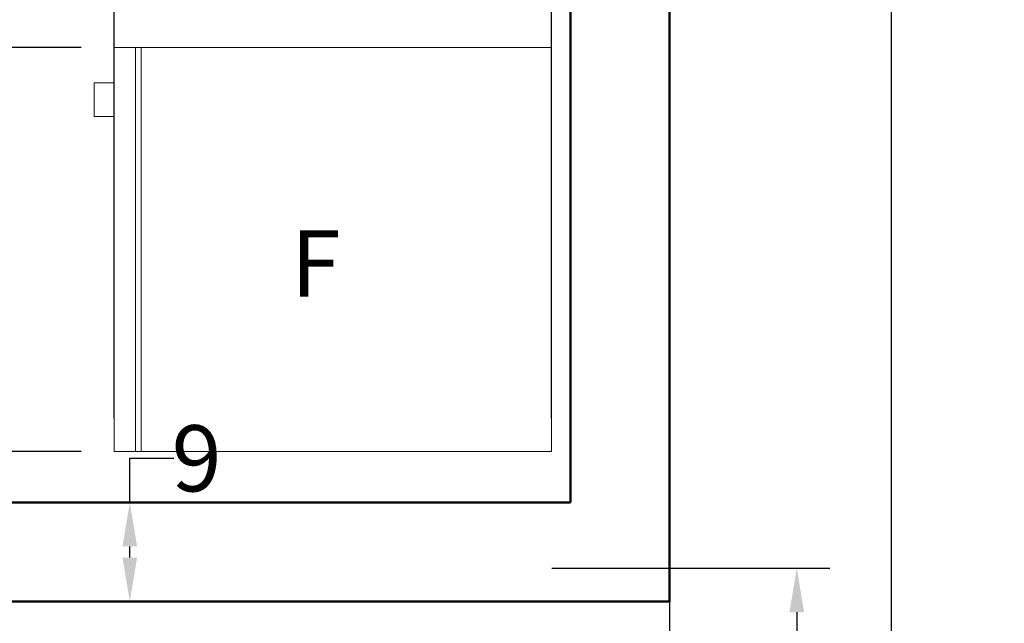
# Model space of a CAD drawing. Units: inches. Extents: x 89 to 490, y -59 to 378.
# Tile 17 of 20: x 400 to 490, y 3 to 58. Entities that reach past the tile are written whole.
import ezdxf

# ---------------------------------------------------------------- set-up
doc = ezdxf.new("R2010")
doc.units = ezdxf.units.IN
doc.header["$MEASUREMENT"] = 0
for name, color, linetype, lineweight in [('A-ANNO-DIMS', 2, 'Continuous', 18), ('A-ANNO-TEXT', 7, 'Continuous', 18), ('L-PLNT-EDGE', 31, 'Continuous', 25), ('Outer Walls', 12, 'Continuous', 50), ('Refrigerator', 40, 'Continuous', 18)]:
    doc.layers.add(name, color=color, linetype=linetype, lineweight=lineweight)
doc.styles.get("Standard").update_dxf_attribs({"font": 'arial.ttf'})
doc.dimstyles.get("Standard").update_dxf_attribs({"dimtxt": 6, "dimasz": 4, "dimexe": 3, "dimexo": 3, "dimgap": 0.09, "dimtad": 0, "dimtih": 1, "dimtoh": 1, "dimdec": 1, "dimzin": 0, "dimdsep": 46, "dimlunit": 3, "dimtxsty": 'Standard', "dimcen": 0.09, "dimadec": 0, "dimazin": 0, "dimtfac": 1, "dimtdec": 1, "dimtofl": 0, "dimtmove": 0, "dimatfit": 3, "dimfxl": 1, "dimtolj": 1, "dimtzin": 0, "dimarcsym": 0})

# ---------------------------------------------------------------- blocks, each defined once
blk = doc.blocks.new('*D37')
at = {"layer": 'A-ANNO-DIMS', "color": 0, "lineweight": -2, "transparency": 16777216}
for p, q in [((410.454, 13.741), (410.454, 17.741)), ((410.454, 17.741), (414.454, 17.741)), ((402.654, 13.741), (413.454, 13.741)), ((410.454, 8.741), (410.454, 9.741)), ((402.654, 4.741), (413.454, 4.741))]:
    blk.add_line(p, q, dxfattribs=at)
at = {"layer": 'A-ANNO-DIMS', "color": 0, "transparency": 16777216}
for points in [[(409.787, 9.741), (411.121, 9.741), (410.454, 13.741)], [(409.787, 8.741), (411.121, 8.741), (410.454, 4.741)]]:
    blk.add_solid(points, dxfattribs=at)
at = {"layer": 'Defpoints', "color": 0, "transparency": 16777216}
for p in [(399.654, 13.741), (410.454, 13.741), (399.654, 4.741)]:
    blk.add_point(p, dxfattribs=at)
at = {"layer": 'A-ANNO-DIMS', "color": 0, "transparency": 16777216, "insert": (416.517, 17.741), "char_height": 6, "attachment_point": 5}
blk.add_mtext('\\A1;9', dxfattribs=at)
blk = doc.blocks.new('*D47')
at = {"layer": 'A-ANNO-DIMS', "color": 0, "lineweight": -2, "transparency": 16777216}
for p, q in [((448.739, 7.78), (473.983, 7.78)), ((470.983, 3.78), (470.983, -5.387)), ((470.983, -20.866), (470.983, -11.698)), ((448.739, -24.866), (473.983, -24.866))]:
    blk.add_line(p, q, dxfattribs=at)
at = {"layer": 'A-ANNO-DIMS', "color": 0, "transparency": 16777216}
for points in [[(470.316, 3.78), (471.65, 3.78), (470.983, 7.78)], [(470.316, -20.866), (471.65, -20.866), (470.983, -24.866)]]:
    blk.add_solid(points, dxfattribs=at)
at = {"layer": 'Defpoints', "color": 0, "transparency": 16777216}
for p in [(445.739, 7.78), (470.983, 7.78), (445.739, -24.866)]:
    blk.add_point(p, dxfattribs=at)
at = {"layer": 'A-ANNO-DIMS', "color": 0, "transparency": 16777216, "insert": (470.983, -8.543), "char_height": 6, "attachment_point": 5}
blk.add_mtext('\\A1;33', dxfattribs=at)
blk = doc.blocks.new('*D48')
at = {"layer": 'A-ANNO-DIMS', "color": 0, "lineweight": -2, "transparency": 16777216}
for p, q in [((127.441, 10.741), (127.441, -49.809)), ((459.441, -29.659), (459.441, -49.809)), ((131.441, -46.809), (286.756, -46.809)), ((455.441, -46.809), (300.127, -46.809))]:
    blk.add_line(p, q, dxfattribs=at)
at = {"layer": 'A-ANNO-DIMS', "color": 0, "transparency": 16777216}
for points in [[(131.441, -46.143), (131.441, -47.476), (127.441, -46.809)], [(455.441, -46.143), (455.441, -47.476), (459.441, -46.809)]]:
    blk.add_solid(points, dxfattribs=at)
at = {"layer": 'Defpoints', "color": 0, "transparency": 16777216}
for p in [(127.441, 13.741), (459.441, -26.659), (459.441, -46.809)]:
    blk.add_point(p, dxfattribs=at)
at = {"layer": 'A-ANNO-DIMS', "color": 0, "transparency": 16777216, "insert": (293.441, -46.809), "char_height": 6, "attachment_point": 5}
blk.add_mtext('\\A1;332', dxfattribs=at)
blk = doc.blocks.new('*D49')
at = {"layer": 'A-ANNO-DIMS', "color": 0, "lineweight": -2, "transparency": 16777216}
for p, q in [((462.441, 353.741), (482.591, 353.741)), ((479.591, 349.741), (479.591, 166.696)), ((479.591, -22.659), (479.591, 160.385)), ((462.441, -26.659), (482.591, -26.659))]:
    blk.add_line(p, q, dxfattribs=at)
at = {"layer": 'A-ANNO-DIMS', "color": 0, "transparency": 16777216}
for points in [[(478.925, 349.741), (480.258, 349.741), (479.591, 353.741)], [(478.925, -22.659), (480.258, -22.659), (479.591, -26.659)]]:
    blk.add_solid(points, dxfattribs=at)
at = {"layer": 'Defpoints', "color": 0, "transparency": 16777216}
for p in [(459.441, 353.741), (479.591, 353.741), (459.441, -26.659)]:
    blk.add_point(p, dxfattribs=at)
at = {"layer": 'A-ANNO-DIMS', "color": 0, "transparency": 16777216, "insert": (479.591, 163.541), "char_height": 6, "attachment_point": 5}
blk.add_mtext('\\A1;380.4', dxfattribs=at)
blk = doc.blocks.new('*D64')
at = {"layer": 'A-ANNO-DIMS', "color": 0, "lineweight": -2, "transparency": 16777216}
for p, q in [((399.654, 16.741), (399.654, 376.891)), ((450.441, 16.741), (450.441, 376.891)), ((403.654, 373.891), (414.828, 373.891)), ((446.441, 373.891), (435.267, 373.891))]:
    blk.add_line(p, q, dxfattribs=at)
at = {"layer": 'A-ANNO-DIMS', "color": 0, "transparency": 16777216}
for points in [[(403.654, 374.558), (403.654, 373.225), (399.654, 373.891)], [(446.441, 374.558), (446.441, 373.225), (450.441, 373.891)]]:
    blk.add_solid(points, dxfattribs=at)
at = {"layer": 'Defpoints', "color": 0, "transparency": 16777216}
for p in [(450.441, 373.891), (399.654, 13.741), (450.441, 13.741)]:
    blk.add_point(p, dxfattribs=at)
at = {"layer": 'A-ANNO-DIMS', "color": 0, "transparency": 16777216, "insert": (425.048, 373.891), "char_height": 6, "attachment_point": 5}
blk.add_mtext('\\A1;50.79', dxfattribs=at)
blk = doc.blocks.new('*D71')
at = {"layer": 'A-ANNO-DIMS', "color": 0, "lineweight": -2, "transparency": 16777216}
for p, q in [((409.039, 21.374), (409.039, 376.891)), ((448.723, 21.374), (448.723, 376.891)), ((413.039, 373.891), (416.351, 373.891)), ((444.723, 373.891), (441.411, 373.891))]:
    blk.add_line(p, q, dxfattribs=at)
at = {"layer": 'A-ANNO-DIMS', "color": 0, "transparency": 16777216}
for points in [[(413.039, 374.558), (413.039, 373.225), (409.039, 373.891)], [(444.723, 374.558), (444.723, 373.225), (448.723, 373.891)]]:
    blk.add_solid(points, dxfattribs=at)
at = {"layer": 'Defpoints', "color": 0, "transparency": 16777216}
for p in [(448.723, 373.891), (409.039, 18.374), (448.723, 18.374)]:
    blk.add_point(p, dxfattribs=at)
at = {"layer": 'A-ANNO-DIMS', "color": 0, "transparency": 16777216, "insert": (428.881, 373.891), "char_height": 6, "attachment_point": 5}
blk.add_mtext('\\A1;39.684', dxfattribs=at)
blk = doc.blocks.new('*D72')
at = {"layer": 'A-ANNO-DIMS', "color": 0, "lineweight": -2, "transparency": 16777216}
for p, q in [((406.039, 55.006), (385.889, 55.006)), ((388.889, 51.006), (388.889, 39.845)), ((388.889, 22.374), (388.889, 33.534)), ((406.039, 18.374), (385.889, 18.374))]:
    blk.add_line(p, q, dxfattribs=at)
at = {"layer": 'A-ANNO-DIMS', "color": 0, "transparency": 16777216}
for points in [[(388.222, 51.006), (389.555, 51.006), (388.889, 55.006)], [(388.222, 22.374), (389.555, 22.374), (388.889, 18.374)]]:
    blk.add_solid(points, dxfattribs=at)
at = {"layer": 'Defpoints', "color": 0, "transparency": 16777216}
for p in [(388.889, 55.006), (409.039, 55.006), (409.039, 18.374)]:
    blk.add_point(p, dxfattribs=at)
at = {"layer": 'A-ANNO-DIMS', "color": 0, "transparency": 16777216, "insert": (388.889, 36.69), "char_height": 6, "attachment_point": 5}
blk.add_mtext('\\A1;36.63', dxfattribs=at)

msp = doc.modelspace()

# ---------------------------------------------------------------- linework, layer by layer
at = {"layer": 'L-PLNT-EDGE'}
msp.add_line((459.4414, 12.3406), (459.4414, -26.6594), dxfattribs=at)
at = {"layer": 'Outer Walls'}
for p, q in [((450.4414, 13.7413), (450.4414, 195.7413)), ((270.4414, 13.7413), (450.4414, 13.7413))]:
    msp.add_line(p, q, dxfattribs=at)
msp.add_lwpolyline([(214.6478, 67.7413), (265.4414, 67.7413), (265.4414, 4.7413), (459.4414, 4.7413), (459.4414, 353.7413), (127.4414, 353.7413), (127.4414, 13.7413)], dxfattribs=at)
at = {"layer": 'Refrigerator'}
for p, q in [((410.973, 18.3742), (410.973, 55.0057)), ((411.4809, 18.3742), (411.4809, 55.0057))]:
    msp.add_line(p, q, dxfattribs=at)
msp.add_lwpolyline([(448.7229, 55.0057), (448.7229, 18.3742), (409.0388, 18.3742), (409.0388, 55.0057)], close=True, dxfattribs=at)
msp.add_lwpolyline([(409.0388, 48.7515), (407.2072, 48.7515), (407.2072, 51.8041), (409.0388, 51.8041)], dxfattribs=at)

# ---------------------------------------------------------------- texts
at = {"layer": 'A-ANNO-TEXT', "insert": (425.065, 38.4229), "char_height": 6, "attachment_point": 1}
msp.add_mtext_dynamic_manual_height_columns('F', width=23.657961, gutter_width=1, heights=[0], dxfattribs=at)

# ---------------------------------------------------------------- dimensions: what is measured, and where the dimension line sits
at = {"layer": 'A-ANNO-DIMS'}
for base, p1, p2, override, picture, middle in [((450.4414, 373.8913), (399.6539, 13.7413), (450.4414, 13.7413), {"dimdec": 2, "dimlfac": 1, "dimrnd": 0, "dimzin": 0, "dimdsep": 46, "dimlunit": 2}, '*D64', (425.0477, 373.8913)), ((448.7229, 373.8913), (409.0388, 18.3742), (448.7229, 18.3742), {"dimdec": 3, "dimlfac": 1, "dimrnd": 0, "dimzin": 0, "dimdsep": 46, "dimlunit": 2}, '*D71', (428.8809, 373.8913)), ((459.4414, -46.8094), (127.4414, 13.7413), (459.4414, -26.6594), {"dimdec": 0, "dimlfac": 1, "dimrnd": 0, "dimzin": 0, "dimdsep": 46, "dimlunit": 2}, '*D48', (293.4414, -46.8094))]:
    dim = msp.add_linear_dim(base=base, p1=p1, p2=p2, dimstyle='Standard', override=override, dxfattribs=at)
    dim.commit()
    dim.dimension.update_dxf_attribs({"geometry": picture, "text_midpoint": middle})
for base, p1, p2, override, picture, middle in [((479.5914, 353.7413), (459.4414, -26.6594), (459.4414, 353.7413), {"dimdec": 1, "dimlfac": 1, "dimrnd": 0, "dimzin": 0, "dimdsep": 46, "dimlunit": 2}, '*D49', (479.5914, 163.5409)), ((388.8888, 55.0057), (409.0388, 18.3742), (409.0388, 55.0057), {"dimdec": 2, "dimlfac": 1, "dimrnd": 0, "dimzin": 0, "dimdsep": 46, "dimlunit": 2}, '*D72', (388.8888, 36.69)), ((410.4539, 13.7413), (399.6539, 4.7413), (399.6539, 13.7413), {"dimdec": 0, "dimlfac": 1, "dimrnd": 0, "dimzin": 0, "dimdsep": 46, "dimlunit": 2}, '*D37', (416.5166, 17.7413)), ((470.9829, 7.78), (445.7386, -24.8656), (445.7386, 7.78), {"dimdec": 0, "dimlfac": 1, "dimrnd": 0, "dimzin": 0, "dimdsep": 46, "dimlunit": 2}, '*D47', (470.9829, -8.5428))]:
    dim = msp.add_linear_dim(base=base, p1=p1, p2=p2, angle=90, dimstyle='Standard', override=override, dxfattribs=at)
    dim.commit()
    dim.dimension.update_dxf_attribs({"geometry": picture, "text_midpoint": middle})

doc.saveas('drawing.dxf')
